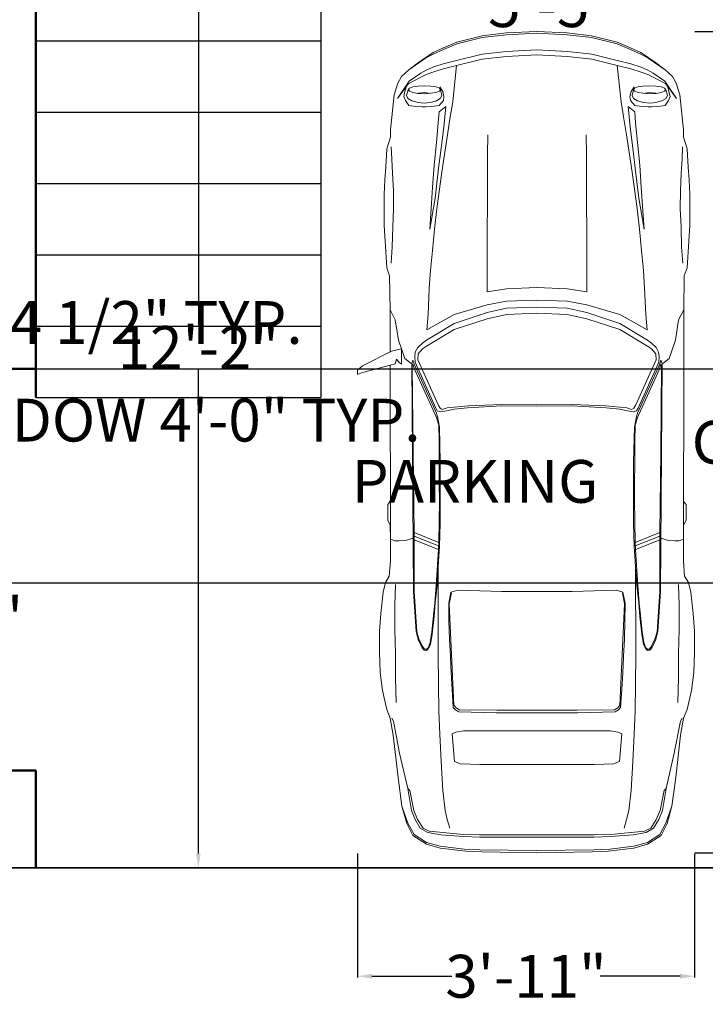
# Model space of a CAD drawing. Units: inches. Extents: x 134 to 568, y 15 to 554.
# Tile 3 of 7: x 415 to 511, y 25 to 164. Entities that reach past the tile are written whole.
import ezdxf

# ---------------------------------------------------------------- set-up
doc = ezdxf.new("R2010")
doc.units = ezdxf.units.IN
doc.header["$MEASUREMENT"] = 0
for name, color, linetype, lineweight in [('A-ANNO-DIMS', 2, 'Continuous', 18), ('A-AREA-IDEN', 7, 'Continuous', 25), ('A-FLOR-STRS', 3, 'Continuous', 25), ('A-SITE-VEHI', 8, 'Continuous', 13), ('A-WALL', 7, 'Continuous', 50), ('C-PROP', 7, 'Continuous', 35)]:
    doc.layers.add(name, color=color, linetype=linetype, lineweight=lineweight)
doc.styles.get("Standard").update_dxf_attribs({"font": 'arial.ttf'})
doc.dimstyles.get("Standard").update_dxf_attribs({"dimtxt": 6, "dimasz": 2, "dimexe": 0.18, "dimexo": 0.0625, "dimgap": 0.09, "dimtad": 0, "dimtih": 1, "dimtoh": 1, "dimdec": 0, "dimzin": 0, "dimdsep": 46, "dimlunit": 4, "dimtxsty": 'Standard', "dimcen": 0.09, "dimadec": 0, "dimazin": 0, "dimtfac": 1, "dimtdec": 0, "dimtofl": 0, "dimtmove": 0, "dimatfit": 3, "dimfxl": 1, "dimtolj": 1, "dimtzin": 0, "dimarcsym": 0})

# ---------------------------------------------------------------- blocks, each defined once
blk = doc.blocks.new('*D2')
at = {"layer": 'A-ANNO-DIMS', "color": 0, "lineweight": -2, "transparency": 16777216}
for p, q in [((457.08, 190.52), (457.08, 165.33)), ((522.08, 190.52), (522.08, 165.33)), ((459.08, 165.51), (481.52, 165.51)), ((520.08, 165.51), (497.65, 165.51))]:
    blk.add_line(p, q, dxfattribs=at)
at = {"layer": 'A-ANNO-DIMS', "color": 0, "transparency": 16777216}
for points in [[(459.08, 165.84), (459.08, 165.18), (457.08, 165.51)], [(520.08, 165.84), (520.08, 165.18), (522.08, 165.51)]]:
    blk.add_solid(points, dxfattribs=at)
at = {"layer": 'Defpoints', "color": 0, "transparency": 16777216}
for p in [(457.08, 190.58), (522.08, 190.58), (522.08, 165.51)]:
    blk.add_point(p, dxfattribs=at)
at = {"layer": 'A-ANNO-DIMS', "color": 0, "transparency": 16777216, "insert": (489.58, 165.51), "char_height": 6, "attachment_point": 5}
blk.add_mtext('\\A1;5\'-5"', dxfattribs=at)
blk = doc.blocks.new('*D6')
at = {"layer": 'A-ANNO-DIMS', "color": 0, "lineweight": -2, "transparency": 16777216}
for p, q in [((522.02, 190.58), (439.72, 190.58)), ((439.9, 188.58), (439.9, 120.68)), ((439.9, 46.58), (439.9, 114.48)), ((522.02, 44.58), (439.72, 44.58))]:
    blk.add_line(p, q, dxfattribs=at)
at = {"layer": 'A-ANNO-DIMS', "color": 0, "transparency": 16777216}
for points in [[(439.57, 188.58), (440.23, 188.58), (439.9, 190.58)], [(439.57, 46.58), (440.23, 46.58), (439.9, 44.58)]]:
    blk.add_solid(points, dxfattribs=at)
at = {"layer": 'Defpoints', "color": 0, "transparency": 16777216}
for p in [(439.9, 190.58), (522.08, 190.58), (522.08, 44.58)]:
    blk.add_point(p, dxfattribs=at)
at = {"layer": 'A-ANNO-DIMS', "color": 0, "transparency": 16777216, "insert": (439.9, 117.58), "char_height": 6, "attachment_point": 5}
blk.add_mtext('\\A1;12\'-2"', dxfattribs=at)
blk = doc.blocks.new('*D11')
at = {"layer": 'A-ANNO-DIMS', "color": 0, "lineweight": -2, "transparency": 16777216}
for p, q in [((417.02, 114.58), (403.83, 114.58)), ((404.01, 112.58), (404.01, 82.74)), ((404.01, 46.58), (404.01, 76.43)), ((412.52, 44.58), (403.83, 44.58))]:
    blk.add_line(p, q, dxfattribs=at)
at = {"layer": 'A-ANNO-DIMS', "color": 0, "transparency": 16777216}
for points in [[(403.67, 112.58), (404.34, 112.58), (404.01, 114.58)], [(403.67, 46.58), (404.34, 46.58), (404.01, 44.58)]]:
    blk.add_solid(points, dxfattribs=at)
at = {"layer": 'Defpoints', "color": 0, "transparency": 16777216}
for p in [(404.01, 114.58), (417.08, 114.58), (412.58, 44.58)]:
    blk.add_point(p, dxfattribs=at)
at = {"layer": 'A-ANNO-DIMS', "color": 0, "transparency": 16777216, "insert": (404.01, 79.58), "char_height": 6, "attachment_point": 5}
blk.add_mtext('\\A1;5\'-10"', dxfattribs=at)
blk = doc.blocks.new('dsfdhgjk')
at = {"color": 0, "linetype": 'ByBlock'}
for p, q in [((392.31, -140.4, -279.43), (388.73, -141.3, -279.43)), ((392.31, -140.66, -279.43), (388.73, -141.55, -279.43)), ((395.72, -140.02, -279.43), (392.31, -140.4, -279.43)), ((395.72, -140.27, -279.43), (392.31, -140.66, -279.43)), ((399.98, -139.81, -279.43), (395.72, -140.02, -279.43)), ((399.98, -140.05, -279.43), (395.72, -140.27, -279.43)), ((399.98, -139.81, -279.43), (399.98, -139.81, -279.43)), ((399.98, -139.81, -279.43), (404.24, -140.02, -279.43)), ((399.98, -140.05, -279.43), (404.24, -140.27, -279.43)), ((404.24, -140.02, -279.43), (407.65, -140.4, -279.43)), ((404.24, -140.27, -279.43), (407.65, -140.66, -279.43)), ((407.65, -140.4, -279.43), (411.24, -141.3, -279.43)), ((407.65, -140.66, -279.43), (411.24, -141.55, -279.43)), ((386.85, -142.1, -279.43), (385.4, -142.74, -279.43)), ((388.73, -141.3, -279.43), (386.85, -142.1, -279.43)), ((388.73, -141.55, -279.43), (386.85, -142.36, -279.43)), ((411.24, -141.3, -279.43), (413.11, -142.1, -279.43)), ((411.24, -141.55, -279.43), (413.11, -142.36, -279.43)), ((413.11, -142.1, -279.43), (414.57, -142.74, -279.43)), ((384.37, -143.55, -279.43), (381.99, -145.17, -279.43)), ((385.4, -142.74, -279.43), (383.36, -144.15, -279.43)), ((385.4, -143, -279.43), (384.37, -143.55, -279.43)), ((386.85, -142.36, -279.43), (385.4, -143, -279.43)), ((388.71, -143.89, -279.43), (392.3, -143, -279.43)), ((392.3, -143, -279.43), (395.71, -142.61, -279.43)), ((395.71, -143.3, -279.43), (392.3, -143.68, -279.43)), ((395.71, -142.61, -279.43), (399.98, -142.4, -279.43)), ((399.98, -143.09, -279.43), (395.71, -143.3, -279.43)), ((404.25, -142.61, -279.43), (399.98, -142.4, -279.43)), ((399.98, -143.09, -279.43), (404.25, -143.3, -279.43)), ((407.67, -143, -279.43), (404.25, -142.61, -279.43)), ((404.25, -143.3, -279.43), (407.67, -143.68, -279.43)), ((411.25, -143.89, -279.43), (407.67, -143, -279.43)), ((413.11, -142.36, -279.43), (414.57, -143, -279.43)), ((414.57, -142.74, -279.43), (416.61, -144.15, -279.43)), ((414.57, -143, -279.43), (415.59, -143.55, -279.43)), ((415.59, -143.55, -279.43), (417.98, -145.17, -279.43)), ((383.36, -144.15, -279.43), (381.99, -145.17, -279.43)), ((384.44, -145.25, -279.43), (385.38, -144.83, -279.43)), ((385.38, -144.83, -279.43), (386.84, -144.37, -279.43)), ((386.84, -144.37, -279.43), (388.71, -143.89, -279.43)), ((388.71, -144.58, -279.43), (386.84, -145.04, -279.43)), ((388.71, -144.58, -279.43), (388.18, -149.68, -279.43)), ((392.3, -143.68, -279.43), (388.71, -144.58, -279.43)), ((407.67, -143.68, -279.43), (411.25, -144.58, -279.43)), ((413.13, -144.37, -279.43), (411.25, -143.89, -279.43)), ((411.25, -144.58, -279.43), (413.13, -145.04, -279.43)), ((411.25, -144.58, -279.43), (411.79, -149.68, -279.43)), ((414.58, -144.83, -279.43), (413.13, -144.37, -279.43)), ((415.52, -145.25, -279.43), (414.58, -144.83, -279.43)), ((416.61, -144.15, -279.43), (417.98, -145.17, -279.43)), ((380.96, -146.12, -279.43), (380.45, -147.05, -279.43)), ((381.99, -145.17, -279.43), (380.96, -146.12, -279.43)), ((383.69, -146.2, -279.43), (381.9, -147.14, -279.43)), ((382.06, -146.79, -279.43), (383.69, -145.68, -279.43)), ((383.69, -145.68, -279.43), (384.44, -145.25, -279.43)), ((384.44, -145.86, -279.43), (383.69, -146.2, -279.43)), ((385.38, -145.51, -279.43), (384.44, -145.86, -279.43)), ((386.84, -145.04, -279.43), (385.38, -145.51, -279.43)), ((413.13, -145.04, -279.43), (414.58, -145.51, -279.43)), ((414.58, -145.51, -279.43), (415.52, -145.86, -279.43)), ((416.28, -145.68, -279.43), (415.52, -145.25, -279.43)), ((415.52, -145.86, -279.43), (416.28, -146.2, -279.43)), ((417.91, -146.79, -279.43), (416.28, -145.68, -279.43)), ((416.28, -146.2, -279.43), (418.06, -147.14, -279.43)), ((417.98, -145.17, -279.43), (419, -146.12, -279.43)), ((419, -146.12, -279.43), (419.52, -147.05, -279.43)), ((380.45, -147.05, -279.43), (379.94, -148.68, -279.43)), ((380.41, -149.2, -279.43), (382.06, -146.79, -279.43)), ((381.9, -147.14, -279.43), (380.41, -149.2, -279.43)), ((381.65, -147.56, -279.43), (381.47, -148.25, -279.43)), ((382.08, -147.77, -279.43), (381.9, -147.99, -279.43)), ((382.58, -147.59, -279.43), (382.08, -147.77, -279.43)), ((383.32, -147.47, -279.43), (382.58, -147.59, -279.43)), ((384.21, -147.43, -279.43), (383.32, -147.47, -279.43)), ((385.08, -147.47, -279.43), (384.21, -147.43, -279.43)), ((385.84, -147.59, -279.43), (385.08, -147.47, -279.43)), ((386.3, -147.77, -279.43), (385.84, -147.59, -279.43)), ((386.46, -147.99, -279.43), (386.3, -147.77, -279.43)), ((386.77, -148.25, -279.43), (386.34, -147.56, -279.43)), ((413.2, -148.25, -279.43), (413.63, -147.56, -279.43)), ((413.51, -147.99, -279.43), (413.66, -147.77, -279.43)), ((413.66, -147.77, -279.43), (414.13, -147.59, -279.43)), ((414.13, -147.59, -279.43), (414.88, -147.47, -279.43)), ((414.88, -147.47, -279.43), (415.76, -147.43, -279.43)), ((415.76, -147.43, -279.43), (416.64, -147.47, -279.43)), ((416.64, -147.47, -279.43), (417.39, -147.59, -279.43)), ((417.39, -147.59, -279.43), (417.89, -147.77, -279.43)), ((417.89, -147.77, -279.43), (418.06, -147.99, -279.43)), ((419.55, -149.2, -279.43), (417.91, -146.79, -279.43)), ((418.06, -147.14, -279.43), (419.55, -149.2, -279.43)), ((418.32, -147.56, -279.43), (418.49, -148.25, -279.43)), ((419.52, -147.05, -279.43), (420.03, -148.68, -279.43)), ((379.94, -148.68, -279.43), (379.42, -153.62, -279.43)), ((381.47, -148.25, -279.43), (381.31, -148.93, -279.43)), ((381.31, -148.93, -279.43), (381.52, -149.5, -279.43)), ((381.66, -148.79, -279.43), (381.9, -147.99, -279.43)), ((381.86, -149.22, -279.43), (381.66, -148.79, -279.43)), ((381.9, -147.99, -279.43), (382.08, -148.19, -279.43)), ((382.08, -148.19, -279.43), (382.58, -148.37, -279.43)), ((382.58, -148.37, -279.43), (383.25, -148.49, -279.43)), ((383.25, -148.49, -279.43), (384.21, -148.55, -279.43)), ((383.32, -148.47, -279.43), (384.21, -148.35, -279.43)), ((384.21, -148.35, -279.43), (385.07, -148.5, -279.43)), ((384.21, -148.55, -279.43), (385.08, -148.47, -279.43)), ((385.08, -148.47, -279.43), (385.78, -148.39, -279.43)), ((385.78, -148.39, -279.43), (386.29, -148.2, -279.43)), ((386.29, -148.2, -279.43), (386.46, -147.99, -279.43)), ((386.64, -148.79, -279.43), (386.42, -149.22, -279.43)), ((386.46, -147.99, -279.43), (386.6, -148.54, -279.43)), ((386.6, -148.54, -279.43), (386.64, -148.79, -279.43)), ((386.93, -148.93, -279.43), (386.77, -148.25, -279.43)), ((386.86, -149.5, -279.43), (386.93, -148.93, -279.43)), ((413.03, -148.93, -279.43), (413.2, -148.25, -279.43)), ((413.1, -149.5, -279.43), (413.03, -148.93, -279.43)), ((413.37, -148.54, -279.43), (413.32, -148.79, -279.43)), ((413.32, -148.79, -279.43), (413.54, -149.22, -279.43)), ((413.51, -147.99, -279.43), (413.37, -148.54, -279.43)), ((413.67, -148.2, -279.43), (413.51, -147.99, -279.43)), ((414.18, -148.39, -279.43), (413.67, -148.2, -279.43)), ((414.88, -148.47, -279.43), (414.18, -148.39, -279.43)), ((415.76, -148.55, -279.43), (414.88, -148.47, -279.43)), ((415.76, -148.35, -279.43), (414.89, -148.5, -279.43)), ((416.64, -148.47, -279.43), (415.76, -148.35, -279.43)), ((416.71, -148.49, -279.43), (415.76, -148.55, -279.43)), ((417.39, -148.37, -279.43), (416.71, -148.49, -279.43)), ((417.89, -148.19, -279.43), (417.39, -148.37, -279.43)), ((418.06, -147.99, -279.43), (417.89, -148.19, -279.43)), ((418.31, -148.79, -279.43), (418.06, -147.99, -279.43)), ((418.11, -149.22, -279.43), (418.31, -148.79, -279.43)), ((418.65, -148.93, -279.43), (418.45, -149.5, -279.43)), ((418.49, -148.25, -279.43), (418.65, -148.93, -279.43)), ((420.03, -148.68, -279.43), (420.54, -153.62, -279.43)), ((381.52, -149.5, -279.43), (381.99, -150.18, -279.43)), ((382.45, -149.56, -279.43), (381.86, -149.22, -279.43)), ((381.99, -150.18, -279.43), (383.01, -150.35, -279.43)), ((383.31, -149.79, -279.43), (382.45, -149.56, -279.43)), ((383.01, -150.35, -279.43), (383.86, -150.39, -279.43)), ((384.16, -149.88, -279.43), (383.31, -149.79, -279.43)), ((383.86, -150.39, -279.43), (384.37, -150.39, -279.43)), ((385.01, -149.79, -279.43), (384.16, -149.88, -279.43)), ((384.37, -150.39, -279.43), (385.23, -150.35, -279.43)), ((385.87, -149.56, -279.43), (385.01, -149.79, -279.43)), ((385.23, -150.35, -279.43), (386.26, -150.18, -279.43)), ((386.42, -149.22, -279.43), (385.87, -149.56, -279.43)), ((386.26, -150.18, -279.43), (386.86, -149.5, -279.43)), ((387.2, -150.33, -279.43), (386.27, -151.1, -279.43)), ((386.9, -153.25, -279.43), (387.2, -150.33, -279.43)), ((388.18, -149.68, -279.43), (387.83, -151.78, -279.43)), ((411.79, -149.68, -279.43), (412.14, -151.78, -279.43)), ((413.07, -153.25, -279.43), (412.76, -150.33, -279.43)), ((412.76, -150.33, -279.43), (413.7, -151.1, -279.43)), ((413.71, -150.18, -279.43), (413.1, -149.5, -279.43)), ((413.54, -149.22, -279.43), (414.09, -149.56, -279.43)), ((414.73, -150.35, -279.43), (413.71, -150.18, -279.43)), ((414.09, -149.56, -279.43), (414.95, -149.79, -279.43)), ((415.59, -150.39, -279.43), (414.73, -150.35, -279.43)), ((414.95, -149.79, -279.43), (415.8, -149.88, -279.43)), ((416.11, -150.39, -279.43), (415.59, -150.39, -279.43)), ((415.8, -149.88, -279.43), (416.65, -149.79, -279.43)), ((416.96, -150.35, -279.43), (416.11, -150.39, -279.43)), ((416.65, -149.79, -279.43), (417.51, -149.56, -279.43)), ((417.98, -150.18, -279.43), (416.96, -150.35, -279.43)), ((417.51, -149.56, -279.43), (418.11, -149.22, -279.43)), ((418.45, -149.5, -279.43), (417.98, -150.18, -279.43)), ((386.27, -151.1, -279.43), (386.14, -152.61, -279.43)), ((387.83, -151.78, -279.43), (387.43, -154.31, -279.43)), ((412.14, -151.78, -279.43), (412.53, -154.31, -279.43)), ((413.7, -151.1, -279.43), (413.82, -152.61, -279.43)), ((386.14, -152.61, -279.43), (385.87, -155.38, -279.43)), ((386.53, -156.17, -279.43), (386.9, -153.25, -279.43)), ((413.44, -156.17, -279.43), (413.07, -153.25, -279.43)), ((413.82, -152.61, -279.43), (414.09, -155.38, -279.43)), ((379.42, -154.65, -279.43), (378.92, -156.27, -279.43)), ((379.42, -153.62, -279.43), (379.42, -154.65, -279.43)), ((387.43, -154.31, -279.43), (387.03, -157.06, -279.43)), ((393.06, -157.06, -279.43), (393.09, -154.31, -279.43)), ((406.91, -157.06, -279.43), (406.87, -154.31, -279.43)), ((412.53, -154.31, -279.43), (412.94, -157.06, -279.43)), ((420.54, -153.62, -279.43), (420.54, -154.65, -279.43)), ((420.54, -154.65, -279.43), (421.04, -156.27, -279.43)), ((379.54, -156.01, -279.43), (379.62, -157.71, -279.43)), ((385.87, -155.38, -279.43), (385.57, -158.55, -279.43)), ((414.09, -155.38, -279.43), (414.39, -158.55, -279.43)), ((420.42, -156.01, -279.43), (420.34, -157.71, -279.43)), ((378.92, -156.27, -279.43), (378.77, -158.83, -279.43)), ((386.19, -159, -279.43), (386.53, -156.17, -279.43)), ((387.03, -157.06, -279.43), (386.62, -159.53, -279.43)), ((393, -174.76, -279.43), (393.06, -157.06, -279.43)), ((406.97, -174.76, -279.43), (406.91, -157.06, -279.43)), ((412.94, -157.06, -279.43), (413.35, -159.53, -279.43)), ((413.78, -159, -279.43), (413.44, -156.17, -279.43)), ((421.04, -156.27, -279.43), (421.19, -158.83, -279.43)), ((379.62, -157.71, -279.43), (379.74, -159.68, -279.43)), ((385.57, -158.55, -279.43), (385.35, -161.71, -279.43)), ((414.39, -158.55, -279.43), (414.62, -161.71, -279.43)), ((420.34, -157.71, -279.43), (420.23, -159.68, -279.43)), ((378.77, -158.83, -279.43), (378.63, -160.62, -279.43)), ((379.74, -159.68, -279.43), (379.86, -162.15, -279.43)), ((385.7, -163.17, -279.43), (386.19, -159, -279.43)), ((386.62, -159.53, -279.43), (385.93, -164.62, -279.43)), ((413.35, -159.53, -279.43), (414.03, -164.62, -279.43)), ((414.27, -163.17, -279.43), (413.78, -159, -279.43)), ((420.23, -159.68, -279.43), (420.11, -162.15, -279.43)), ((421.19, -158.83, -279.43), (421.33, -160.62, -279.43)), ((378.63, -160.62, -279.43), (378.55, -162.66, -279.43)), ((421.33, -160.62, -279.43), (421.41, -162.66, -279.43)), ((378.55, -162.66, -279.43), (378.55, -164.62, -279.43)), ((379.86, -162.15, -279.43), (379.88, -164.62, -279.43)), ((385.35, -161.71, -279.43), (384.97, -167.52, -279.43)), ((414.62, -161.71, -279.43), (415, -167.52, -279.43)), ((420.11, -162.15, -279.43), (420.09, -164.62, -279.43)), ((421.41, -162.66, -279.43), (421.41, -164.62, -279.43)), ((384.97, -167.52, -279.43), (385.7, -163.17, -279.43)), ((415, -167.52, -279.43), (414.27, -163.17, -279.43)), ((378.55, -164.62, -279.43), (378.55, -167.01, -279.43)), ((379.88, -164.62, -279.43), (379.76, -167.23, -279.43)), ((385.93, -164.62, -279.43), (385.59, -167.52, -279.43)), ((414.03, -164.62, -279.43), (414.37, -167.52, -279.43)), ((420.09, -164.62, -279.43), (420.2, -167.23, -279.43)), ((421.41, -164.62, -279.43), (421.41, -167.01, -279.43)), ((378.55, -167.01, -279.43), (378.69, -169.23, -279.43)), ((421.41, -167.01, -279.43), (421.27, -169.23, -279.43)), ((379.76, -167.23, -279.43), (379.68, -170.08, -279.43)), ((385.59, -167.52, -279.43), (385.31, -170.52, -279.43)), ((414.37, -167.52, -279.43), (414.65, -170.52, -279.43)), ((420.2, -167.23, -279.43), (420.28, -170.08, -279.43)), ((378.69, -169.23, -279.43), (378.92, -172.98, -279.43)), ((421.27, -169.23, -279.43), (421.04, -172.98, -279.43)), ((379.68, -170.08, -279.43), (379.52, -172.33, -279.43)), ((385.31, -170.52, -279.43), (385.06, -173.32, -279.43)), ((414.65, -170.52, -279.43), (414.91, -173.32, -279.43)), ((420.28, -170.08, -279.43), (420.45, -172.33, -279.43)), ((378.92, -172.98, -279.43), (379.32, -174.1, -279.43)), ((385.06, -173.32, -279.43), (384.88, -175.8, -279.43)), ((414.91, -173.32, -279.43), (415.08, -175.8, -279.43)), ((421.04, -172.98, -279.43), (420.65, -174.1, -279.43)), ((379.32, -174.1, -279.43), (379.39, -178.87, -279.43)), ((392.99, -176.32, -279.43), (393, -174.76, -279.43)), ((406.98, -176.32, -279.43), (406.97, -174.76, -279.43)), ((420.65, -174.1, -279.43), (420.58, -178.87, -279.43)), ((384.88, -175.8, -279.43), (384.72, -179.49, -279.43)), ((395.72, -175.9, -279.43), (392.99, -176.32, -279.43)), ((399.98, -175.73, -279.43), (395.72, -175.9, -279.43)), ((399.98, -175.73, -279.43), (404.24, -175.9, -279.43)), ((404.24, -175.9, -279.43), (406.98, -176.32, -279.43)), ((415.08, -175.8, -279.43), (415.24, -179.49, -279.43)), ((392.99, -178.16, -279.43), (395.72, -177.65, -279.43)), ((395.72, -177.65, -279.43), (399.98, -177.48, -279.43)), ((404.24, -177.65, -279.43), (399.98, -177.48, -279.43)), ((406.98, -178.16, -279.43), (404.24, -177.65, -279.43)), ((379.39, -178.87, -279.43), (379.38, -184.78, -279.43)), ((380.11, -180.24, -279.43), (379.39, -178.87, -279.43)), ((384.72, -179.49, -279.43), (384.55, -181.64, -279.43)), ((384.55, -181.64, -279.43), (388.38, -179.53, -279.43)), ((388.38, -179.53, -279.43), (392.99, -178.16, -279.43)), ((392.99, -179.23, -279.43), (388.38, -180.77, -279.43)), ((395.72, -178.64, -279.43), (392.99, -179.23, -279.43)), ((395.72, -179.5, -279.43), (392.99, -180.1, -279.43)), ((399.98, -178.47, -279.43), (395.72, -178.64, -279.43)), ((399.98, -179.33, -279.43), (395.72, -179.5, -279.43)), ((399.98, -178.47, -279.43), (404.24, -178.64, -279.43)), ((399.98, -179.33, -279.43), (404.24, -179.5, -279.43)), ((404.24, -178.64, -279.43), (406.98, -179.23, -279.43)), ((404.24, -179.5, -279.43), (406.98, -180.1, -279.43)), ((411.59, -179.53, -279.43), (406.98, -178.16, -279.43)), ((406.98, -179.23, -279.43), (411.59, -180.77, -279.43)), ((415.42, -181.64, -279.43), (411.59, -179.53, -279.43)), ((415.24, -179.49, -279.43), (415.42, -181.64, -279.43)), ((419.85, -180.24, -279.43), (420.58, -178.87, -279.43)), ((420.58, -178.87, -279.43), (420.59, -184.78, -279.43)), ((380.57, -183.13, -279.43), (380.11, -180.24, -279.43)), ((388.38, -180.77, -279.43), (384.47, -183.13, -279.43)), ((392.99, -180.1, -279.43), (388.38, -181.63, -279.43)), ((406.98, -180.1, -279.43), (411.59, -181.63, -279.43)), ((411.59, -180.77, -279.43), (415.5, -183.13, -279.43)), ((419.4, -183.13, -279.43), (419.85, -180.24, -279.43)), ((388.38, -181.63, -279.43), (384.47, -183.96, -279.43)), ((411.59, -181.63, -279.43), (415.5, -183.96, -279.43)), ((381.43, -185.69, -279.43), (380.57, -183.13, -279.43)), ((383.91, -183.54, -279.43), (383.27, -184.16, -279.43)), ((384.47, -183.13, -279.43), (383.91, -183.54, -279.43)), ((415.5, -183.13, -279.43), (416.06, -183.54, -279.43)), ((416.06, -183.54, -279.43), (416.7, -184.16, -279.43)), ((418.54, -185.69, -279.43), (419.4, -183.13, -279.43)), ((379.6, -184.67, -279.43), (375.5, -186.72, -279.43)), ((380.96, -184.33, -279.43), (379.6, -184.67, -279.43)), ((380.96, -186.46, -279.43), (380.96, -184.33, -279.43)), ((382.92, -184.8, -279.43), (382.86, -185.47, -279.43)), ((383.27, -184.16, -279.43), (382.92, -184.8, -279.43)), ((383.31, -185.02, -279.43), (383.25, -185.89, -279.43)), ((383.91, -184.33, -279.43), (383.31, -185.02, -279.43)), ((384.47, -183.96, -279.43), (383.91, -184.33, -279.43)), ((415.5, -183.96, -279.43), (416.06, -184.33, -279.43)), ((416.06, -184.33, -279.43), (416.65, -185.02, -279.43)), ((416.65, -185.02, -279.43), (416.71, -185.89, -279.43)), ((416.7, -184.16, -279.43), (417.05, -184.8, -279.43)), ((417.05, -184.8, -279.43), (417.11, -185.47, -279.43)), ((420.58, -186.61, -279.43), (420.59, -184.78, -279.43)), ((379.4, -186.61, -279.43), (380.11, -186.44, -279.43)), ((380.11, -186.44, -279.43), (380.29, -185.78, -279.43)), ((380.29, -185.78, -279.43), (380.69, -186.28, -279.43)), ((380.69, -186.28, -279.43), (380.96, -186.46, -279.43)), ((382.35, -186.38, -279.43), (381.43, -185.69, -279.43)), ((382.42, -186.38, -279.43), (382.59, -185.9, -279.43)), ((382.66, -218.37, -279.43), (382.42, -186.38, -279.43)), ((382.59, -185.9, -279.43), (382.81, -186.57, -279.43)), ((382.86, -185.47, -279.43), (382.88, -186.21, -279.43)), ((382.88, -186.21, -279.43), (385.8, -192.63, -279.43)), ((383.25, -185.89, -279.43), (386.15, -192.28, -279.43)), ((416.71, -185.89, -279.43), (413.81, -192.28, -279.43)), ((417.08, -186.21, -279.43), (414.16, -192.63, -279.43)), ((417.11, -185.47, -279.43), (417.08, -186.21, -279.43)), ((417.37, -185.9, -279.43), (417.15, -186.57, -279.43)), ((417.3, -218.37, -279.43), (417.55, -186.38, -279.43)), ((417.55, -186.38, -279.43), (417.37, -185.9, -279.43)), ((417.62, -186.38, -279.43), (418.54, -185.69, -279.43)), ((375.5, -186.72, -279.43), (374.83, -187.31, -279.43)), ((374.83, -187.31, -279.43), (374.83, -187.91, -279.43)), ((374.83, -187.91, -279.43), (375.5, -187.65, -279.43)), ((375.5, -187.65, -279.43), (379.4, -186.61, -279.43)), ((379.39, -186.61, -279.43), (379.44, -211.03, -279.43)), ((382.5, -186.75, -279.43), (382.59, -186.5, -279.43)), ((382.63, -198.85, -279.43), (382.5, -186.75, -279.43)), ((382.59, -186.5, -279.43), (382.81, -187.17, -279.43)), ((382.81, -186.57, -279.43), (385.71, -192.92, -279.43)), ((382.81, -187.17, -279.43), (385.71, -193.53, -279.43)), ((417.15, -186.57, -279.43), (414.25, -192.92, -279.43)), ((417.15, -187.17, -279.43), (414.25, -193.53, -279.43)), ((417.37, -186.5, -279.43), (417.15, -187.17, -279.43)), ((417.34, -198.85, -279.43), (417.47, -186.75, -279.43)), ((417.47, -186.75, -279.43), (417.37, -186.5, -279.43)), ((420.58, -186.61, -279.43), (420.53, -211.03, -279.43)), ((385.71, -192.92, -279.43), (385.87, -193.35, -279.43)), ((385.8, -192.63, -279.43), (386, -193.02, -279.43)), ((386, -193.02, -279.43), (386.5, -193.18, -279.43)), ((386.15, -192.28, -279.43), (386.39, -192.67, -279.43)), ((386.39, -192.67, -279.43), (386.7, -192.82, -279.43)), ((386.5, -193.18, -279.43), (387.31, -193.02, -279.43)), ((386.7, -192.82, -279.43), (387.4, -192.62, -279.43)), ((387.31, -193.02, -279.43), (388.38, -192.81, -279.43)), ((387.4, -192.62, -279.43), (390.32, -192.32, -279.43)), ((388.38, -192.81, -279.43), (390.26, -192.59, -279.43)), ((390.26, -192.59, -279.43), (395.05, -192.34, -279.43)), ((390.32, -192.32, -279.43), (395.05, -192.13, -279.43)), ((395.05, -192.13, -279.43), (399.98, -192.1, -279.43)), ((395.05, -192.34, -279.43), (399.98, -192.37, -279.43)), ((404.92, -192.13, -279.43), (399.98, -192.1, -279.43)), ((404.92, -192.34, -279.43), (399.98, -192.37, -279.43)), ((409.64, -192.32, -279.43), (404.92, -192.13, -279.43)), ((409.7, -192.59, -279.43), (404.92, -192.34, -279.43)), ((412.57, -192.62, -279.43), (409.64, -192.32, -279.43)), ((411.59, -192.81, -279.43), (409.7, -192.59, -279.43)), ((412.66, -193.02, -279.43), (411.59, -192.81, -279.43)), ((413.26, -192.82, -279.43), (412.57, -192.62, -279.43)), ((413.46, -193.18, -279.43), (412.66, -193.02, -279.43)), ((413.58, -192.67, -279.43), (413.26, -192.82, -279.43)), ((413.96, -193.02, -279.43), (413.46, -193.18, -279.43)), ((413.81, -192.28, -279.43), (413.58, -192.67, -279.43)), ((414.16, -192.63, -279.43), (413.96, -193.02, -279.43)), ((414.25, -192.92, -279.43), (414.09, -193.35, -279.43)), ((385.71, -193.53, -279.43), (385.87, -193.96, -279.43)), ((385.87, -193.35, -279.43), (386.04, -193.82, -279.43)), ((385.87, -193.96, -279.43), (386.04, -194.43, -279.43)), ((386.04, -193.82, -279.43), (386.3, -195.3, -279.43)), ((386.04, -194.43, -279.43), (386.2, -195.05, -279.43)), ((413.93, -193.82, -279.43), (413.66, -195.3, -279.43)), ((413.93, -194.43, -279.43), (413.77, -195.05, -279.43)), ((414.09, -193.35, -279.43), (413.93, -193.82, -279.43)), ((414.09, -193.96, -279.43), (413.93, -194.43, -279.43)), ((414.25, -193.53, -279.43), (414.09, -193.96, -279.43)), ((386.2, -195.05, -279.43), (386.27, -197.25, -279.43)), ((386.3, -195.3, -279.43), (386.42, -200.2, -279.43)), ((413.66, -195.3, -279.43), (413.54, -200.2, -279.43)), ((413.77, -195.05, -279.43), (413.7, -197.25, -279.43)), ((386.27, -197.25, -279.43), (386.27, -200.19, -279.43)), ((413.7, -197.25, -279.43), (413.7, -200.19, -279.43)), ((382.75, -210.09, -279.43), (382.63, -198.85, -279.43)), ((417.21, -210.09, -279.43), (417.34, -198.85, -279.43)), ((386.27, -200.19, -279.43), (386.28, -203.3, -279.43)), ((386.42, -200.2, -279.43), (386.42, -205.57, -279.43)), ((413.54, -200.2, -279.43), (413.54, -205.57, -279.43)), ((413.7, -200.19, -279.43), (413.68, -203.3, -279.43)), ((386.28, -203.3, -279.43), (386.3, -205.58, -279.43)), ((413.68, -203.3, -279.43), (413.66, -205.58, -279.43)), ((379.41, -205.74, -279.43), (379.08, -206.17, -279.43)), ((379.41, -205.57, -279.43), (379.41, -205.74, -279.43)), ((386.3, -205.58, -279.43), (386.21, -211.48, -279.43)), ((386.42, -205.57, -279.43), (386.42, -208.78, -279.43)), ((413.54, -205.57, -279.43), (413.54, -208.78, -279.43)), ((413.66, -205.58, -279.43), (413.75, -211.48, -279.43)), ((420.55, -205.57, -279.43), (420.55, -205.74, -279.43)), ((420.55, -205.74, -279.43), (420.89, -206.17, -279.43)), ((379.08, -206.17, -279.43), (379.08, -208.38, -279.43)), ((420.89, -206.17, -279.43), (420.89, -208.38, -279.43)), ((379.08, -208.38, -279.43), (379.41, -209.07, -279.43)), ((420.89, -208.38, -279.43), (420.55, -209.07, -279.43)), ((379.41, -209.07, -279.43), (379.41, -210, -279.43)), ((386.42, -208.78, -279.43), (386.33, -212.04, -279.43)), ((413.54, -208.78, -279.43), (413.63, -212.04, -279.43)), ((420.55, -209.07, -279.43), (420.55, -210, -279.43)), ((379.44, -211.03, -279.43), (379.42, -214.04, -279.43)), ((380.08, -211.28, -279.43), (379.44, -211.03, -279.43)), ((380.6, -211.28, -279.43), (380.08, -211.28, -279.43)), ((381.55, -211.2, -279.43), (380.6, -211.28, -279.43)), ((382.42, -210.94, -279.43), (381.55, -211.2, -279.43)), ((382.75, -210.94, -279.43), (382.42, -210.94, -279.43)), ((382.74, -218.37, -279.43), (382.75, -210.94, -279.43)), ((382.75, -210.09, -279.43), (386.21, -211.48, -279.43)), ((382.75, -210.94, -279.43), (382.75, -210.09, -279.43)), ((382.75, -210.6, -279.43), (386.19, -211.98, -279.43)), ((382.75, -211.1, -279.43), (386.16, -212.47, -279.43)), ((417.21, -210.09, -279.43), (413.75, -211.48, -279.43)), ((417.21, -210.6, -279.43), (413.78, -211.98, -279.43)), ((417.21, -211.1, -279.43), (413.8, -212.47, -279.43)), ((417.21, -210.94, -279.43), (417.21, -210.09, -279.43)), ((417.22, -218.37, -279.43), (417.21, -210.94, -279.43)), ((417.21, -210.94, -279.43), (417.55, -210.94, -279.43)), ((417.55, -210.94, -279.43), (418.41, -211.2, -279.43)), ((418.41, -211.2, -279.43), (419.36, -211.28, -279.43)), ((419.36, -211.28, -279.43), (419.89, -211.28, -279.43)), ((419.89, -211.28, -279.43), (420.53, -211.03, -279.43)), ((420.53, -211.03, -279.43), (420.54, -214.04, -279.43)), ((386.16, -212.48, -279.43), (385.83, -217.51, -279.43)), ((386.33, -212.04, -279.43), (386.14, -214.87, -279.43)), ((386.21, -211.48, -279.43), (386.16, -212.48, -279.43)), ((413.63, -212.04, -279.43), (413.82, -214.87, -279.43)), ((413.75, -211.48, -279.43), (413.8, -212.48, -279.43)), ((413.8, -212.48, -279.43), (414.14, -217.51, -279.43)), ((379.42, -214.04, -279.43), (379.26, -216.23, -279.43)), ((420.54, -214.04, -279.43), (420.7, -216.23, -279.43)), ((386.14, -214.87, -279.43), (385.97, -217.51, -279.43)), ((386.14, -214.87, -279.43), (386.12, -227.07, -279.43)), ((413.82, -214.87, -279.43), (414, -217.51, -279.43)), ((413.82, -214.87, -279.43), (413.85, -227.07, -279.43)), ((379.26, -216.23, -279.43), (378.75, -217.09, -279.43)), ((420.7, -216.23, -279.43), (421.22, -217.09, -279.43)), ((378.75, -217.09, -279.43), (378.41, -218.45, -279.43)), ((380.13, -217.4, -279.43), (380.04, -220.22, -279.43)), ((385.83, -217.51, -279.43), (385.65, -219.99, -279.43)), ((385.97, -217.51, -279.43), (385.72, -219.97, -279.43)), ((388.89, -218.2, -279.43), (387.91, -218.45, -279.43)), ((395.04, -218.36, -279.43), (388.89, -218.2, -279.43)), ((404.93, -218.36, -279.43), (411.08, -218.2, -279.43)), ((411.08, -218.2, -279.43), (412.05, -218.45, -279.43)), ((414, -217.51, -279.43), (414.25, -219.97, -279.43)), ((414.14, -217.51, -279.43), (414.31, -219.99, -279.43)), ((419.84, -217.4, -279.43), (419.93, -220.22, -279.43)), ((421.22, -217.09, -279.43), (421.55, -218.45, -279.43)), ((378.41, -218.45, -279.43), (378.06, -221.43, -279.43)), ((383.03, -223.99, -279.43), (382.66, -218.37, -279.43)), ((383.14, -224.01, -279.43), (382.74, -218.37, -279.43)), ((387.91, -218.45, -279.43), (387.6, -219.98, -279.43)), ((387.69, -220.09, -279.43), (388, -218.57, -279.43)), ((399.99, -218.37, -279.43), (395.04, -218.36, -279.43)), ((399.97, -218.37, -279.43), (404.93, -218.36, -279.43)), ((412.28, -220.09, -279.43), (411.96, -218.57, -279.43)), ((412.05, -218.45, -279.43), (412.37, -219.98, -279.43)), ((416.83, -224.01, -279.43), (417.22, -218.37, -279.43)), ((416.93, -223.99, -279.43), (417.3, -218.37, -279.43)), ((421.55, -218.45, -279.43), (421.9, -221.43, -279.43)), ((380.04, -220.22, -279.43), (380.04, -223.71, -279.43)), ((385.65, -219.99, -279.43), (385.47, -221.67, -279.43)), ((385.72, -219.97, -279.43), (385.55, -221.89, -279.43)), ((387.6, -219.98, -279.43), (387.64, -222.42, -279.43)), ((388.34, -234.33, -279.43), (387.69, -220.09, -279.43)), ((411.62, -234.33, -279.43), (412.28, -220.09, -279.43)), ((412.37, -219.98, -279.43), (412.32, -222.42, -279.43)), ((414.25, -219.97, -279.43), (414.41, -221.89, -279.43)), ((414.31, -219.99, -279.43), (414.5, -221.67, -279.43)), ((419.93, -220.22, -279.43), (419.93, -223.71, -279.43)), ((378.06, -221.43, -279.43), (377.9, -223.91, -279.43)), ((385.47, -221.67, -279.43), (385.23, -224.02, -279.43)), ((385.55, -221.89, -279.43), (385.27, -224.34, -279.43)), ((414.41, -221.89, -279.43), (414.69, -224.34, -279.43)), ((414.5, -221.67, -279.43), (414.73, -224.02, -279.43)), ((421.9, -221.43, -279.43), (422.07, -223.91, -279.43)), ((380.04, -223.71, -279.43), (380.13, -227.04, -279.43)), ((387.64, -222.42, -279.43), (387.72, -225.08, -279.43)), ((412.32, -222.42, -279.43), (412.24, -225.08, -279.43)), ((419.93, -223.71, -279.43), (419.84, -227.04, -279.43)), ((377.9, -223.91, -279.43), (377.9, -226.89, -279.43)), ((383.3, -225.09, -279.43), (383.03, -223.99, -279.43)), ((383.43, -225.04, -279.43), (383.14, -224.01, -279.43)), ((383.87, -226.25, -279.43), (383.3, -225.09, -279.43)), ((383.96, -226.14, -279.43), (383.43, -225.04, -279.43)), ((385.23, -224.02, -279.43), (384.99, -225.54, -279.43)), ((385.27, -224.34, -279.43), (385.03, -225.79, -279.43)), ((387.72, -225.08, -279.43), (387.84, -227.43, -279.43)), ((412.24, -225.08, -279.43), (412.12, -227.43, -279.43)), ((414.69, -224.34, -279.43), (414.94, -225.79, -279.43)), ((414.73, -224.02, -279.43), (414.98, -225.54, -279.43)), ((416, -226.14, -279.43), (416.54, -225.04, -279.43)), ((416.09, -226.25, -279.43), (416.66, -225.09, -279.43)), ((416.54, -225.04, -279.43), (416.83, -224.01, -279.43)), ((416.66, -225.09, -279.43), (416.93, -223.99, -279.43)), ((422.07, -223.91, -279.43), (422.07, -226.89, -279.43)), ((384.14, -226.6, -279.43), (383.87, -226.25, -279.43)), ((384.22, -226.44, -279.43), (383.96, -226.14, -279.43)), ((384.5, -226.45, -279.43), (384.22, -226.44, -279.43)), ((384.72, -226.4, -279.43), (384.49, -226.64, -279.43)), ((384.72, -226.28, -279.43), (384.5, -226.45, -279.43)), ((384.99, -225.54, -279.43), (384.72, -226.28, -279.43)), ((385.03, -225.79, -279.43), (384.72, -226.4, -279.43)), ((414.94, -225.79, -279.43), (415.24, -226.4, -279.43)), ((414.98, -225.54, -279.43), (415.24, -226.28, -279.43)), ((415.24, -226.28, -279.43), (415.47, -226.45, -279.43)), ((415.24, -226.4, -279.43), (415.48, -226.64, -279.43)), ((415.47, -226.45, -279.43), (415.74, -226.44, -279.43)), ((415.74, -226.44, -279.43), (416, -226.14, -279.43)), ((415.83, -226.6, -279.43), (416.09, -226.25, -279.43)), ((377.9, -226.89, -279.43), (377.98, -229.71, -279.43)), ((380.13, -227.04, -279.43), (380.13, -230.49, -279.43)), ((384.49, -226.64, -279.43), (384.14, -226.6, -279.43)), ((386.12, -227.07, -279.43), (386.16, -231.42, -279.43)), ((387.84, -227.43, -279.43), (387.89, -228.79, -279.43)), ((412.12, -227.43, -279.43), (412.08, -228.79, -279.43)), ((413.85, -227.07, -279.43), (413.8, -231.42, -279.43)), ((415.48, -226.64, -279.43), (415.83, -226.6, -279.43)), ((419.84, -227.04, -279.43), (419.84, -230.49, -279.43)), ((422.07, -226.89, -279.43), (421.98, -229.71, -279.43)), ((387.89, -228.79, -279.43), (387.99, -230.55, -279.43)), ((412.08, -228.79, -279.43), (411.97, -230.55, -279.43)), ((377.98, -229.71, -279.43), (378.32, -232.27, -279.43)), ((380.13, -230.49, -279.43), (380.22, -233.95, -279.43)), ((387.99, -230.55, -279.43), (388.09, -232.11, -279.43)), ((411.97, -230.55, -279.43), (411.88, -232.11, -279.43)), ((419.84, -230.49, -279.43), (419.74, -233.95, -279.43)), ((421.98, -229.71, -279.43), (421.65, -232.27, -279.43)), ((386.16, -231.42, -279.43), (386.21, -235.17, -279.43)), ((413.8, -231.42, -279.43), (413.75, -235.17, -279.43)), ((378.32, -232.27, -279.43), (378.91, -234.91, -279.43)), ((388.09, -232.11, -279.43), (388.25, -234.62, -279.43)), ((411.88, -232.11, -279.43), (411.72, -234.62, -279.43)), ((421.65, -232.27, -279.43), (421.05, -234.91, -279.43)), ((388.25, -234.62, -279.43), (388.55, -234.98, -279.43)), ((388.63, -234.69, -279.43), (388.34, -234.33, -279.43)), ((389.1, -234.96, -279.43), (388.63, -234.69, -279.43)), ((410.87, -234.96, -279.43), (411.33, -234.69, -279.43)), ((411.33, -234.69, -279.43), (411.62, -234.33, -279.43)), ((411.72, -234.62, -279.43), (411.41, -234.98, -279.43)), ((378.91, -234.91, -279.43), (379.4, -236.11, -279.43)), ((379.4, -236.11, -279.43), (379.82, -238.5, -279.43)), ((379.63, -236.11, -279.43), (379.87, -236.53, -279.43)), ((386.21, -235.17, -279.43), (386.35, -238.36, -279.43)), ((388.55, -234.98, -279.43), (389.01, -235.26, -279.43)), ((389.01, -235.26, -279.43), (394.28, -235.36, -279.43)), ((394.36, -235.02, -279.43), (389.1, -234.96, -279.43)), ((394.28, -235.36, -279.43), (399.98, -235.36, -279.43)), ((399.99, -235.02, -279.43), (394.36, -235.02, -279.43)), ((399.97, -235.02, -279.43), (405.61, -235.02, -279.43)), ((405.69, -235.36, -279.43), (399.98, -235.36, -279.43)), ((405.61, -235.02, -279.43), (410.87, -234.96, -279.43)), ((410.96, -235.26, -279.43), (405.69, -235.36, -279.43)), ((411.41, -234.98, -279.43), (410.96, -235.26, -279.43)), ((413.75, -235.17, -279.43), (413.61, -238.36, -279.43)), ((420.33, -236.11, -279.43), (420.1, -236.53, -279.43)), ((420.56, -236.11, -279.43), (420.14, -238.5, -279.43)), ((421.05, -234.91, -279.43), (420.56, -236.11, -279.43)), ((379.87, -236.53, -279.43), (380.72, -241.02, -279.43)), ((420.1, -236.53, -279.43), (419.25, -241.02, -279.43)), ((379.82, -238.5, -279.43), (380.52, -244.47, -279.43)), ((386.35, -238.36, -279.43), (386.53, -242.19, -279.43)), ((388.07, -238.35, -279.43), (388.62, -238.09, -279.43)), ((388.41, -242.2, -279.43), (388.07, -238.35, -279.43)), ((388.62, -238.09, -279.43), (389.66, -237.92, -279.43)), ((389.66, -237.92, -279.43), (394.28, -237.89, -279.43)), ((394.28, -237.89, -279.43), (399.98, -237.89, -279.43)), ((405.69, -237.89, -279.43), (399.98, -237.89, -279.43)), ((410.31, -237.92, -279.43), (405.69, -237.89, -279.43)), ((411.34, -238.09, -279.43), (410.31, -237.92, -279.43)), ((411.89, -238.35, -279.43), (411.34, -238.09, -279.43)), ((411.55, -242.2, -279.43), (411.89, -238.35, -279.43)), ((413.61, -238.36, -279.43), (413.44, -242.19, -279.43)), ((420.14, -238.5, -279.43), (419.45, -244.47, -279.43)), ((380.72, -241.02, -279.43), (381.85, -246.01, -279.43)), ((419.25, -241.02, -279.43), (418.12, -246.01, -279.43)), ((386.53, -242.19, -279.43), (386.76, -246.26, -279.43)), ((389.24, -242.53, -279.43), (388.41, -242.2, -279.43)), ((391.97, -242.62, -279.43), (389.24, -242.53, -279.43)), ((399.98, -242.62, -279.43), (391.97, -242.62, -279.43)), ((399.98, -242.62, -279.43), (407.99, -242.62, -279.43)), ((407.99, -242.62, -279.43), (410.73, -242.53, -279.43)), ((410.73, -242.53, -279.43), (411.55, -242.2, -279.43)), ((413.44, -242.19, -279.43), (413.21, -246.26, -279.43)), ((380.52, -244.47, -279.43), (381.05, -248.47, -279.43)), ((419.45, -244.47, -279.43), (418.91, -248.47, -279.43)), ((381.85, -246.01, -279.43), (382.14, -246.26, -279.43)), ((381.85, -246.01, -279.43), (382.37, -249.08, -279.43)), ((382.14, -246.26, -279.43), (382.72, -249.08, -279.43)), ((386.76, -246.26, -279.43), (387.12, -249.08, -279.43)), ((413.21, -246.26, -279.43), (412.85, -249.08, -279.43)), ((417.83, -246.26, -279.43), (417.25, -249.08, -279.43)), ((418.12, -246.01, -279.43), (417.6, -249.08, -279.43)), ((418.12, -246.01, -279.43), (417.83, -246.26, -279.43)), ((381.72, -250.91, -279.43), (381.05, -248.47, -279.43)), ((381.05, -248.47, -279.43), (381.88, -250.86, -279.43)), ((418.91, -248.47, -279.43), (418.08, -250.86, -279.43)), ((418.24, -250.91, -279.43), (418.91, -248.47, -279.43)), ((382.37, -249.08, -279.43), (382.89, -250.35, -279.43)), ((382.72, -249.08, -279.43), (383.24, -250.35, -279.43)), ((387.12, -249.08, -279.43), (387.41, -250.35, -279.43)), ((412.85, -249.08, -279.43), (412.55, -250.35, -279.43)), ((417.25, -249.08, -279.43), (416.72, -250.35, -279.43)), ((417.6, -249.08, -279.43), (417.07, -250.35, -279.43)), ((382.58, -252.57, -279.43), (381.72, -250.91, -279.43)), ((381.88, -250.86, -279.43), (382.74, -252.47, -279.43)), ((382.89, -250.35, -279.43), (383.62, -251.55, -279.43)), ((383.24, -250.35, -279.43), (384.01, -251.55, -279.43)), ((387.41, -250.35, -279.43), (387.76, -251.55, -279.43)), ((412.55, -250.35, -279.43), (412.21, -251.55, -279.43)), ((416.72, -250.35, -279.43), (415.95, -251.55, -279.43)), ((417.07, -250.35, -279.43), (416.35, -251.55, -279.43)), ((418.08, -250.86, -279.43), (417.22, -252.47, -279.43)), ((417.39, -252.57, -279.43), (418.24, -250.91, -279.43)), ((384.47, -253.82, -279.43), (382.58, -252.57, -279.43)), ((382.74, -252.47, -279.43), (384.47, -253.56, -279.43)), ((383.62, -251.55, -279.43), (384.67, -252.19, -279.43)), ((384.01, -251.55, -279.43), (384.88, -251.98, -279.43)), ((384.67, -252.19, -279.43), (386.48, -252.51, -279.43)), ((384.88, -251.98, -279.43), (389.64, -252.46, -279.43)), ((386.48, -252.51, -279.43), (389.67, -252.72, -279.43)), ((389.64, -252.46, -279.43), (391.94, -252.5, -279.43)), ((389.67, -252.72, -279.43), (391.96, -252.81, -279.43)), ((408.03, -252.5, -279.43), (391.94, -252.5, -279.43)), ((410.3, -252.72, -279.43), (408, -252.81, -279.43)), ((410.33, -252.46, -279.43), (408.03, -252.5, -279.43)), ((413.49, -252.51, -279.43), (410.3, -252.72, -279.43)), ((415.08, -251.98, -279.43), (410.33, -252.46, -279.43)), ((415.29, -252.19, -279.43), (413.49, -252.51, -279.43)), ((415.95, -251.55, -279.43), (415.08, -251.98, -279.43)), ((416.35, -251.55, -279.43), (415.29, -252.19, -279.43)), ((417.22, -252.47, -279.43), (415.5, -253.56, -279.43)), ((415.5, -253.82, -279.43), (417.39, -252.57, -279.43)), ((384.47, -253.56, -279.43), (386.4, -254.1, -279.43)), ((386.4, -254.35, -279.43), (384.47, -253.82, -279.43)), ((386.4, -254.1, -279.43), (389.76, -254.52, -279.43)), ((391.96, -252.81, -279.43), (408, -252.81, -279.43)), ((413.57, -254.1, -279.43), (410.2, -254.52, -279.43)), ((415.5, -253.56, -279.43), (413.57, -254.1, -279.43)), ((413.57, -254.35, -279.43), (415.5, -253.82, -279.43)), ((390.02, -254.8, -279.43), (386.4, -254.35, -279.43)), ((389.76, -254.52, -279.43), (391.99, -254.61, -279.43)), ((392.24, -254.89, -279.43), (390.02, -254.8, -279.43)), ((391.99, -254.61, -279.43), (399.98, -254.7, -279.43)), ((399.97, -255.04, -279.43), (392.24, -254.89, -279.43)), ((407.98, -254.61, -279.43), (399.98, -254.7, -279.43)), ((399.99, -255.04, -279.43), (407.72, -254.89, -279.43)), ((407.72, -254.89, -279.43), (409.95, -254.8, -279.43)), ((410.2, -254.52, -279.43), (407.98, -254.61, -279.43)), ((409.95, -254.8, -279.43), (413.57, -254.35, -279.43))]:
    blk.add_line(p, q, dxfattribs=at)
blk = doc.blocks.new('*D50')
at = {"layer": 'A-ANNO-DIMS', "color": 0, "lineweight": -2, "transparency": 16777216}
for p, q in [((346.58, 114.52), (346.58, 107.2)), ((394.58, 114.52), (394.58, 107.2)), ((348.58, 107.38), (392.58, 107.38)), ((394.58, 107.38), (396.58, 107.38))]:
    blk.add_line(p, q, dxfattribs=at)
at = {"layer": 'A-ANNO-DIMS', "color": 0, "transparency": 16777216}
for points in [[(348.58, 107.72), (348.58, 107.05), (346.58, 107.38)], [(392.58, 107.72), (392.58, 107.05), (394.58, 107.38)]]:
    blk.add_solid(points, dxfattribs=at)
at = {"layer": 'Defpoints', "color": 0, "transparency": 16777216}
for p in [(346.58, 114.58), (394.58, 114.58), (394.58, 107.38)]:
    blk.add_point(p, dxfattribs=at)
at = {"layer": 'A-ANNO-DIMS', "color": 0, "transparency": 16777216, "insert": (434.64, 107.38), "char_height": 6, "attachment_point": 5}
blk.add_mtext('\\A1;WINDOW 4\'-0" TYP.', dxfattribs=at)
blk = doc.blocks.new('*D51')
at = {"layer": 'A-ANNO-DIMS', "color": 0, "lineweight": -2, "transparency": 16777216}
for p, q in [((401.78, 119.08), (401.78, 121.08)), ((401.78, 121.08), (403.78, 121.08)), ((394.65, 119.08), (401.96, 119.08)), ((401.78, 116.58), (401.78, 117.08)), ((394.65, 114.58), (401.96, 114.58))]:
    blk.add_line(p, q, dxfattribs=at)
at = {"layer": 'A-ANNO-DIMS', "color": 0, "transparency": 16777216}
for points in [[(401.45, 117.08), (402.12, 117.08), (401.78, 119.08)], [(401.45, 116.58), (402.12, 116.58), (401.78, 114.58)]]:
    blk.add_solid(points, dxfattribs=at)
at = {"layer": 'Defpoints', "color": 0, "transparency": 16777216}
for p in [(394.58, 119.08), (401.78, 119.08), (394.58, 114.58)]:
    blk.add_point(p, dxfattribs=at)
at = {"layer": 'A-ANNO-DIMS', "color": 0, "transparency": 16777216, "insert": (429.15, 121.08), "char_height": 6, "attachment_point": 5}
blk.add_mtext('\\A1;0\'-4 1/2" TYP.', dxfattribs=at)
blk = doc.blocks.new('*D56')
at = {"layer": 'A-ANNO-DIMS', "color": 0, "lineweight": -2, "transparency": 16777216}
for p, q in [((509.54, 161.9), (526.94, 161.9)), ((526.76, 159.9), (526.76, 107.47)), ((526.76, 48.67), (526.76, 101.09)), ((509.54, 46.67), (526.94, 46.67))]:
    blk.add_line(p, q, dxfattribs=at)
at = {"layer": 'A-ANNO-DIMS', "color": 0, "transparency": 16777216}
for points in [[(526.43, 159.9), (527.09, 159.9), (526.76, 161.9)], [(526.43, 48.67), (527.09, 48.67), (526.76, 46.67)]]:
    blk.add_solid(points, dxfattribs=at)
at = {"layer": 'Defpoints', "color": 0, "transparency": 16777216}
for p in [(509.48, 161.9), (526.76, 161.9), (509.48, 46.67)]:
    blk.add_point(p, dxfattribs=at)
at = {"layer": 'A-ANNO-DIMS', "color": 0, "transparency": 16777216, "insert": (526.76, 104.28), "char_height": 6, "attachment_point": 5}
blk.add_mtext('\\A1;CAR 9\'-7"', dxfattribs=at)
blk = doc.blocks.new('*D57')
at = {"layer": 'A-ANNO-DIMS', "color": 0, "lineweight": -2, "transparency": 16777216}
for p, q in [((462.24, 46.6), (462.24, 29.2)), ((509.48, 46.6), (509.48, 29.2)), ((464.24, 29.38), (475.46, 29.38)), ((507.48, 29.38), (496.25, 29.38))]:
    blk.add_line(p, q, dxfattribs=at)
at = {"layer": 'A-ANNO-DIMS', "color": 0, "transparency": 16777216}
for points in [[(464.24, 29.71), (464.24, 29.05), (462.24, 29.38)], [(507.48, 29.71), (507.48, 29.05), (509.48, 29.38)]]:
    blk.add_solid(points, dxfattribs=at)
at = {"layer": 'Defpoints', "color": 0, "transparency": 16777216}
for p in [(462.24, 46.67), (509.48, 46.67), (509.48, 29.38)]:
    blk.add_point(p, dxfattribs=at)
at = {"layer": 'A-ANNO-DIMS', "color": 0, "transparency": 16777216, "insert": (485.86, 29.38), "char_height": 6, "attachment_point": 5}
blk.add_mtext('\\A1;3\'-11"', dxfattribs=at)
blk = doc.blocks.new('*D62')
at = {"layer": 'A-ANNO-DIMS', "color": 0, "lineweight": -2, "transparency": 16777216}
for p, q in [((346.65, 114.58), (556.81, 114.58)), ((556.63, 112.58), (556.63, 102.74)), ((556.63, 86.58), (556.63, 96.43)), ((346.65, 84.58), (556.81, 84.58))]:
    blk.add_line(p, q, dxfattribs=at)
at = {"layer": 'A-ANNO-DIMS', "color": 0, "transparency": 16777216}
for points in [[(556.3, 112.58), (556.97, 112.58), (556.63, 114.58)], [(556.3, 86.58), (556.97, 86.58), (556.63, 84.58)]]:
    blk.add_solid(points, dxfattribs=at)
at = {"layer": 'Defpoints', "color": 0, "transparency": 16777216}
for p in [(346.58, 114.58), (556.63, 114.58), (346.58, 84.58)]:
    blk.add_point(p, dxfattribs=at)
at = {"layer": 'A-ANNO-DIMS', "color": 0, "transparency": 16777216, "insert": (556.63, 99.58), "char_height": 6, "attachment_point": 5}
blk.add_mtext('\\A1;2\'-6"', dxfattribs=at)

msp = doc.modelspace()

# ---------------------------------------------------------------- linework, layer by layer
at = {"layer": 'A-FLOR-STRS'}
for p, q in [((457.08, 230.58), (457.08, 110.58)), ((417.08, 160.58), (457.08, 160.58)), ((417.08, 150.58), (457.08, 150.58)), ((417.08, 140.58), (457.08, 140.58)), ((417.08, 130.58), (457.08, 130.58)), ((417.08, 120.58), (457.08, 120.58)), ((417.08, 110.58), (457.08, 110.58))]:
    msp.add_line(p, q, dxfattribs=at)
at = {"layer": 'A-WALL'}
for p, q in [((417.08, 230.58), (417.08, 110.58)), ((340.58, 114.58), (417.08, 114.58)), ((417.08, 58.26), (412.58, 58.26)), ((417.08, 44.58), (417.08, 58.26))]:
    msp.add_line(p, q, dxfattribs=at)
at = {"layer": 'C-PROP'}
msp.add_line((171.08, 44.58), (531.08, 44.58), dxfattribs=at)

# ---------------------------------------------------------------- block references
at = {"layer": 'A-SITE-VEHI'}
msp.add_blockref('dsfdhgjk', (87.41, 301.71, 279.43), dxfattribs=at)

# ---------------------------------------------------------------- texts
at = {"layer": 'A-AREA-IDEN', "insert": (456.25, 101.79), "char_height": 6, "attachment_point": 1}
msp.add_mtext_dynamic_manual_height_columns('\\pxqc;PARKING', width=44.9119, gutter_width=30, heights=[0], dxfattribs=at)

# ---------------------------------------------------------------- dimensions: what is measured, and where the dimension line sits
at = {"layer": 'A-ANNO-DIMS'}
for base, p1, p2, override, picture, middle in [((439.9, 190.58), (522.08, 44.58), (522.08, 190.58), {"dimclrd": 0, "dimclre": 0, "dimclrt": 0}, '*D6', (439.9, 117.58)), ((556.63, 114.58), (346.58, 84.58), (346.58, 114.58), {"dimdec": 1, "dimlfac": 1, "dimrnd": 0, "dimzin": 1, "dimdsep": 46, "dimlunit": 4, "dimfrac": 2}, '*D62', (556.63, 99.58)), ((404.01, 114.58), (412.58, 44.58), (417.08, 114.58), {"dimclrd": 0, "dimclre": 0, "dimclrt": 0}, '*D11', (404.01, 79.58))]:
    dim = msp.add_linear_dim(base=base, p1=p1, p2=p2, angle=90, dimstyle='Standard', override=override, dxfattribs=at)
    dim.commit()
    dim.dimension.update_dxf_attribs({"geometry": picture, "text_midpoint": middle})
for base, p1, p2, override, picture, middle in [((522.08, 165.51), (457.08, 190.58), (522.08, 190.58), {"dimclrd": 0, "dimclre": 0, "dimclrt": 0}, '*D2', (489.58, 165.51)), ((509.48, 29.38), (462.24, 46.67), (509.48, 46.67), {"dimdec": 1, "dimlfac": 1, "dimrnd": 0, "dimzin": 1, "dimdsep": 46, "dimlunit": 4, "dimfrac": 2}, '*D57', (485.86, 29.38))]:
    dim = msp.add_linear_dim(base=base, p1=p1, p2=p2, dimstyle='Standard', override=override, dxfattribs=at)
    dim.commit()
    dim.dimension.update_dxf_attribs({"geometry": picture, "text_midpoint": middle})
for base, p1, p2, text, picture, middle in [((526.76, 161.9), (509.48, 46.67), (509.48, 161.9), 'CAR <>', '*D56', (526.76, 104.28)), ((401.78, 119.08), (394.58, 114.58), (394.58, 119.08), '<> TYP.', '*D51', (429.15, 121.08))]:
    dim = msp.add_linear_dim(base=base, p1=p1, p2=p2, angle=90, text=text, dimstyle='Standard', override={"dimdec": 1, "dimlfac": 1, "dimrnd": 0, "dimzin": 1, "dimdsep": 46, "dimlunit": 4, "dimfrac": 2}, dxfattribs=at)
    dim.commit()
    dim.dimension.update_dxf_attribs({"geometry": picture, "text_midpoint": middle})
dim = msp.add_linear_dim(base=(394.58, 107.38), p1=(346.58, 114.58), p2=(394.58, 114.58), text='WINDOW <> TYP.', dimstyle='Standard', override={"dimdec": 1, "dimlfac": 1, "dimrnd": 0, "dimzin": 1, "dimdsep": 46, "dimlunit": 4, "dimfrac": 2}, dxfattribs=at)
dim.commit()
dim.dimension.update_dxf_attribs({"geometry": '*D50', "text_midpoint": (434.64, 107.38)})

doc.saveas('drawing.dxf')
